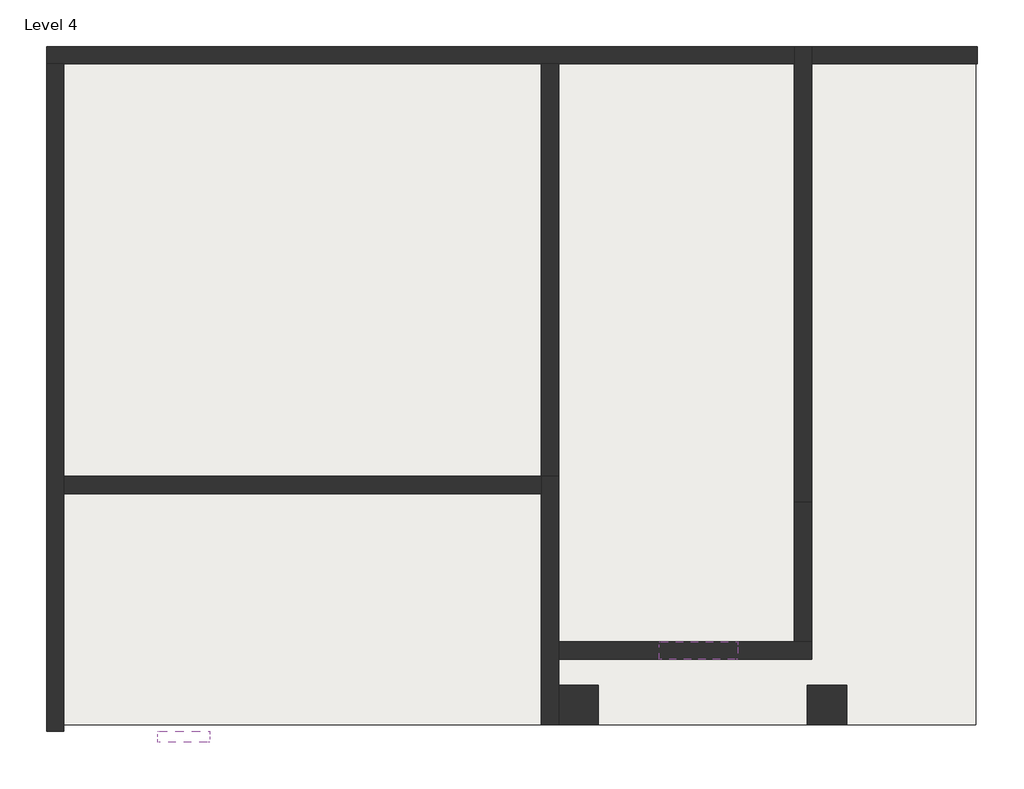
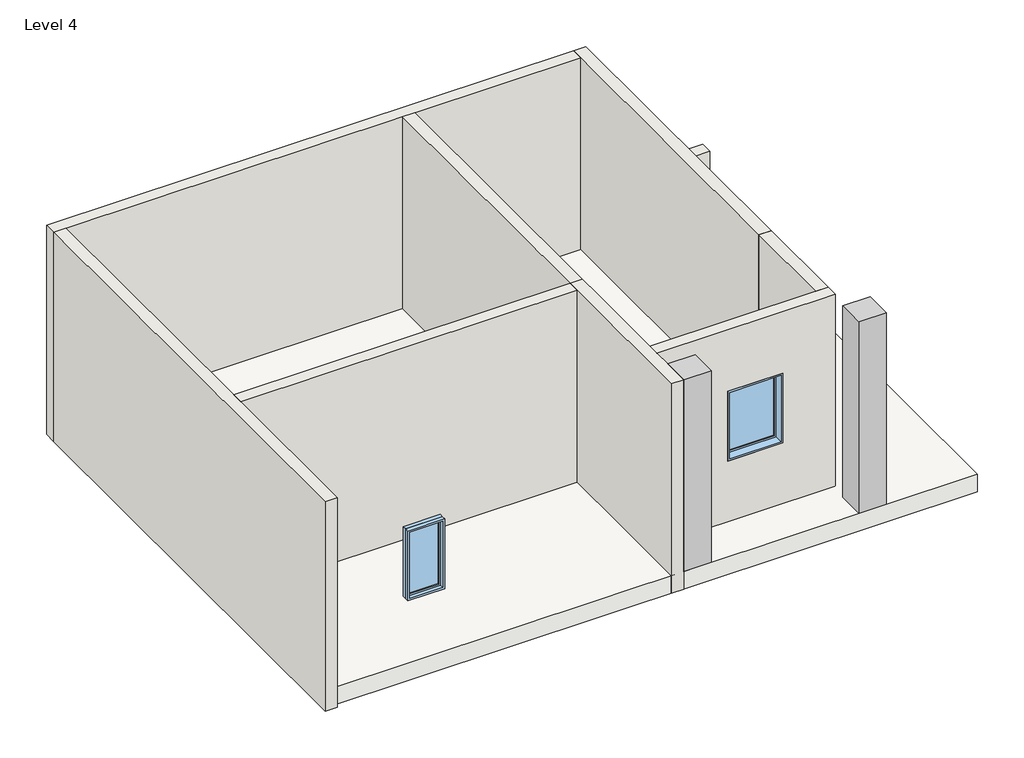
# One storey: 9 walls, 2 columns, 2 windows, 1 roof.
"""IFC4 building model written with IfcOpenShell, lengths in millimetres."""

from ifc_helpers import new_model, si_unit, frame, origin, place, context, project, spatial, polyline, outline, extrude, faceted_brep, transform, mapped, element, save
from components import window_4879aceb, window_e2841890

model = new_model("IFC4")

# Units and contexts
model_context = context("Model", 3, world=origin())
ifc_project = project(units=[si_unit("LENGTHUNIT", "METRE", prefix="MILLI")], contexts=[model_context])

# Site, building, storey
site = spatial("IfcSite", under=ifc_project)
building = spatial("IfcBuilding", under=site)
storey = spatial("IfcBuildingStorey", under=building, Name="Level 4", Elevation=10972.8)

# Columns
placement = place(None, origin())
element("IfcColumn", 1, ObjectType="Rectangular Column : 18\" x 18\"", at=placement, inside=storey, context=model_context, shape_type="SweptSolid", body=[
    extrude(outline(polyline([(-4893.9304753, 3516.0297737), (-4893.9304753, 3058.8297737), (-5351.1304753, 3058.8297737), (-5351.1304753, 3516.0297737), (-4893.9304753, 3516.0297737)])), frame((0.0, 0.0, 11277.6), z_axis=(0.0, 0.0, 1.0), x_axis=(1.0, 0.0, 0.0)), (0.0, 0.0, 1.0), 3352.8),
])
element("IfcColumn", 2, ObjectType="Rectangular Column : 18\" x 18\"", at=placement, inside=storey, context=model_context, shape_type="SweptSolid", body=[
    extrude(outline(polyline([(-7789.5304753, 3516.0297737), (-7789.5304753, 3058.8297737), (-8246.7304753, 3058.8297737), (-8246.7304753, 3516.0297737), (-7789.5304753, 3516.0297737)])), frame((0.0, 0.0, 11277.6), z_axis=(0.0, 0.0, 1.0), x_axis=(1.0, 0.0, 0.0)), (0.0, 0.0, 1.0), 3352.8),
])

# Roof
element("IfcRoof", 3, ObjectType="Generic - 12\"", at=placement, inside=storey, context=model_context, shape_type="SweptSolid", body=[
    extrude(outline(polyline([(-14209.7864811, 10932.8297737), (-3389.3864811, 10932.8297737), (-3389.3864811, 3058.8297737), (-14209.7864811, 3058.8297737), (-14209.7864811, 10932.8297737)])), frame((0.0, 0.0, 10972.8), z_axis=(0.0, 0.0, 1.0), x_axis=(1.0, 0.0, 0.0)), (0.0, 0.0, 1.0), 304.8),
])

# Walls
element("IfcWall", 4, ObjectType="Generic - 8\"", at=placement, inside=storey, context=model_context, shape_type="Brep", body=[
    faceted_brep([(-8449.9304753, 5955.2732783, 10972.8), (-8449.9304753, 5752.0732783, 10972.8), (-8449.9304753, 5548.8732783, 10972.8), (-8449.9304753, 3058.8297737, 10972.8), (-8449.9304753, 3058.8297737, 14630.4), (-8449.9304753, 5548.8732783, 14630.4), (-8449.9304753, 5752.0732783, 14630.4), (-8449.9304753, 5955.2732783, 14630.4), (-8246.7304753, 5955.2732783, 10972.8), (-8246.7304753, 5955.2732783, 14630.4), (-8246.7304753, 5548.8732783, 14630.4), (-8246.7304753, 4024.0297737, 14630.4), (-8246.7304753, 3820.8297737, 14630.4), (-8246.7304753, 3516.0297737, 14630.4), (-8246.7304753, 3058.8297737, 14630.4), (-8246.7304753, 3058.8297737, 11277.6), (-8246.7304753, 3058.8297737, 10972.8), (-8246.7304753, 3820.8297737, 10972.8), (-8246.7304753, 4024.0297737, 10972.8), (-8246.7304753, 5548.8732783, 10972.8)], [[[0, 1, 2, 3, 4, 5, 6, 7]], [[8, 9, 10, 11, 12, 13, 14, 15, 16, 17, 18, 19]], [[3, 2, 1, 0, 8, 19, 18, 17, 16]], [[7, 6, 5, 4, 14, 13, 12, 11, 10, 9]], [[4, 3, 16, 15, 14]], [[0, 7, 9, 8]]]),
])
element("IfcWall", 5, ObjectType="Generic - 8\"", at=placement, inside=storey, context=model_context, shape_type="Brep", body=[
    faceted_brep([(-5300.3304753, 5650.4732783, 10972.8), (-5300.3304753, 10958.2297737, 10972.8), (-5300.3304753, 10958.2297737, 11259.6125244), (-5300.3304753, 10958.2297737, 12248.4392493), (-5300.3304753, 10958.2297737, 14630.4), (-5300.3304753, 5650.4732783, 14630.4), (-5503.5304753, 5650.4732783, 10972.8), (-5503.5304753, 5650.4732783, 14630.4), (-5503.5304753, 10755.0297737, 14630.4), (-5503.5304753, 10958.2297737, 14630.4), (-5503.5304753, 10958.2297737, 10972.8), (-5503.5304753, 10755.0297737, 10972.8)], [[[0, 1, 2, 3, 4, 5]], [[6, 7, 8, 9, 10, 11]], [[1, 0, 6, 11, 10]], [[5, 4, 9, 8, 7]], [[0, 5, 7, 6]], [[1, 10, 9, 4, 3, 2]]]),
])
element("IfcWall", 6, ObjectType="Generic - 8\"", at=placement, inside=storey, context=model_context, shape_type="Brep", body=[
    faceted_brep([(-5503.5304753, 10958.2297737, 14630.4), (-5503.5304753, 10958.2297737, 10972.8), (-14212.6992777, 10958.2297737, 10972.8), (-14212.6992777, 10958.2297737, 14630.4), (-5503.5304753, 10755.0297737, 10972.8), (-5503.5304753, 10755.0297737, 14630.4), (-8246.7304753, 10755.0297737, 14630.4), (-8449.9304753, 10755.0297737, 14630.4), (-14009.4992777, 10755.0297737, 14630.4), (-14212.6992777, 10755.0297737, 14630.4), (-14212.6992777, 10755.0297737, 10972.8), (-14009.4992777, 10755.0297737, 10972.8), (-8449.9304753, 10755.0297737, 10972.8), (-8246.7304753, 10755.0297737, 10972.8)], [[[0, 1, 2, 3]], [[4, 5, 6, 7, 8, 9, 10, 11, 12, 13]], [[2, 1, 4, 13, 12, 11, 10]], [[0, 3, 9, 8, 7, 6, 5]], [[3, 2, 10, 9]], [[0, 5, 4, 1]]]),
])
element("IfcWall", 7, ObjectType="Generic - 8\"", at=placement, inside=storey, context=model_context, shape_type="Brep", body=[
    faceted_brep([(-14212.6992777, 10755.0297737, 10972.8), (-14212.6992777, 2982.6297737, 10972.8), (-14212.6992777, 2982.6297737, 14630.4), (-14212.6992777, 10755.0297737, 14630.4), (-14009.4992777, 10755.0297737, 10972.8), (-14009.4992777, 10755.0297737, 14630.4), (-14009.4992777, 5955.2732783, 14630.4), (-14009.4992777, 5752.0732783, 14630.4), (-14009.4992777, 2982.6297737, 14630.4), (-14009.4992777, 2982.6297737, 10972.8), (-14009.4992777, 5752.0732783, 10972.8), (-14009.4992777, 5955.2732783, 10972.8)], [[[0, 1, 2, 3]], [[4, 5, 6, 7, 8, 9, 10, 11]], [[1, 0, 4, 11, 10, 9]], [[3, 2, 8, 7, 6, 5]], [[0, 3, 5, 4]], [[2, 1, 9, 8]]]),
])
element("IfcWall", 8, ObjectType="Generic - 8\"", at=placement, inside=storey, context=model_context, shape_type="SweptSolid", body=[
    extrude(outline(polyline([(-3369.9304753, 10755.0297737), (-5300.3304753, 10755.0297737), (-5300.3304753, 10958.2297737), (-3369.9304753, 10958.2297737), (-3369.9304753, 10755.0297737)])), frame((0.0, 0.0, 11259.6125244), z_axis=(0.0, 0.0, 1.0), x_axis=(1.0, 0.0, 0.0)), (0.0, 0.0, 1.0), 988.8267249),
])
element("IfcWall", 9, ObjectType="Generic - 8\"", at=placement, inside=storey, context=model_context, shape_type="Brep", body=[
    faceted_brep([(-8246.7304753, 3820.8297737, 10972.8), (-5300.3304753, 3820.8297737, 10972.8), (-5300.3304753, 3820.8297737, 14630.4), (-8246.7304753, 3820.8297737, 14630.4), (-6163.9304753, 3820.8297737, 13556.4516796), (-6163.9304753, 3820.8297737, 12337.2516796), (-7078.3304753, 3820.8297737, 12337.2516796), (-7078.3304753, 3820.8297737, 13556.4516796), (-8246.7304753, 4024.0297737, 10972.8), (-8246.7304753, 4024.0297737, 14630.4), (-5503.5304753, 4024.0297737, 14630.4), (-5300.3304753, 4024.0297737, 14630.4), (-5300.3304753, 4024.0297737, 10972.8), (-5503.5304753, 4024.0297737, 10972.8), (-6163.9304753, 4024.0297737, 13556.4516796), (-7078.3304753, 4024.0297737, 13556.4516796), (-7078.3304753, 4024.0297737, 12337.2516796), (-6163.9304753, 4024.0297737, 12337.2516796)], [[[0, 1, 2, 3], [4, 5, 6, 7]], [[8, 9, 10, 11, 12, 13], [14, 15, 16, 17]], [[1, 0, 8, 13, 12]], [[3, 2, 11, 10, 9]], [[0, 3, 9, 8]], [[2, 1, 12, 11]], [[5, 4, 14, 17]], [[6, 5, 17, 16]], [[7, 6, 16, 15]], [[4, 7, 15, 14]]]),
])
element("IfcWall", 10, ObjectType="Generic - 8\"", at=placement, inside=storey, context=model_context, shape_type="SweptSolid", body=[
    extrude(outline(polyline([(-5503.5304753, 4024.0297737), (-5503.5304753, 5650.4732783), (-5300.3304753, 5650.4732783), (-5300.3304753, 4024.0297737), (-5503.5304753, 4024.0297737)])), frame((0.0, 0.0, 10972.8), z_axis=(0.0, 0.0, 1.0), x_axis=(1.0, 0.0, 0.0)), (0.0, 0.0, 1.0), 3657.6),
])
element("IfcWall", 11, ObjectType="Generic - 8\"", at=placement, inside=storey, context=model_context, shape_type="SweptSolid", body=[
    extrude(outline(polyline([(-14009.4992777, 5955.2732783), (-8449.9304753, 5955.2732783), (-8449.9304753, 5752.0732783), (-14009.4992777, 5752.0732783), (-14009.4992777, 5955.2732783)])), frame((0.0, 0.0, 10972.8), z_axis=(0.0, 0.0, 1.0), x_axis=(1.0, 0.0, 0.0)), (0.0, 0.0, 1.0), 3657.6),
])
element("IfcWall", 12, ObjectType="Generic - 8\"", at=placement, inside=storey, context=model_context, shape_type="SweptSolid", body=[
    extrude(outline(polyline([(-8246.7304753, 10755.0297737), (-8246.7304753, 5955.2732783), (-8449.9304753, 5955.2732783), (-8449.9304753, 10755.0297737), (-8246.7304753, 10755.0297737)])), frame((0.0, 0.0, 10972.8), z_axis=(0.0, 0.0, 1.0), x_axis=(1.0, 0.0, 0.0)), (0.0, 0.0, 1.0), 3657.6),
])

# Windows
window_shape = window_4879aceb(model_context)
element("IfcWindow", 13, ObjectType="Fixed : 24\" x 48\"", at=placement, inside=storey, context=model_context, shape_type="MappedRepresentation", body=[
    mapped(window_shape, transform((-12577.4304753, 2919.1297737, 11613.4331892), x_axis=(1.0, 0.0, 0.0), y_axis=(0.0, 1.0, 0.0), z_axis=(0.0, 0.0, 1.0))),
])
window_2_shape = window_e2841890(model_context)
element("IfcWindow", 14, ObjectType="Fixed : 36\" x 48\"", at=placement, inside=storey, context=model_context, shape_type="MappedRepresentation", body=[
    mapped(window_2_shape, transform((-6583.0304753, 3922.4297737, 11422.8516796), x_axis=(1.0, 0.0, 0.0), y_axis=(0.0, 1.0, 0.0), z_axis=(0.0, 0.0, 1.0))),
])

save(model, "model.ifc")

# Revit data of these elements
# Type "Rectangular Column : 18\" x 18\""
#   Assembly Code = "B1010200"
#   Depth = 1' - 6"
#   Offset Base = 0' - 0"
#   Offset Top = 0' - 0"
#   Width = 1' - 6"
#   Material = none
# Type "Generic - 12\""
#   Assembly Code = "B1020"
#   Layers, outside or top first: 1' - 0" no material (function 1)
# Type "Generic - 8\""
#   Assembly Code = "B2010"
#   Layers, outside or top first: 0' - 8" no material (function 1)
# Type "Fixed : 24\" x 48\""
#   Type Mark = "2"
#   Construction Type Id = "GSP4R"
#   Assembly Code = "B2020100"
#   Analytic Construction = "1/8 in Pilkington single glazing"
#   Visual Light Transmittance = 0.9
#   Solar Heat Gain Coefficient = 0.78
#   Heat Transfer Coefficient (U) = 0.6496 BTU/(h·ft²·°F)
#   Height = 4' - 0"
#   Default Sill Height = 3' - 0"
#   Width = 2' - 0"
#   Window Inset = 0' - 0 3/4"
#   Define Thermal Properties by = 1
#   Glass Pane Material = Glass
#   Sash Material = Sash
#   Wall Closure = (empty or 0)
# Type "Fixed : 36\" x 48\""
#   Type Mark = "1"
#   Construction Type Id = "GSP4R"
#   Assembly Code = "B2020100"
#   Analytic Construction = "1/8 in Pilkington single glazing"
#   Visual Light Transmittance = 0.9
#   Solar Heat Gain Coefficient = 0.78
#   Heat Transfer Coefficient (U) = 0.6496 BTU/(h·ft²·°F)
#   Height = 4' - 0"
#   Default Sill Height = 3' - 0"
#   Width = 3' - 0"
#   Window Inset = 0' - 0 3/4"
#   Define Thermal Properties by = 1
#   Glass Pane Material = Glass
#   Sash Material = Sash
#   Wall Closure = (empty or 0)
# Element 1 (IfcColumn, "Rectangular Column : 18\" x 18\"")
#   Phase Created = New Construction
# Element 2 (IfcColumn, "Rectangular Column : 18\" x 18\"")
#   Phase Created = New Construction
#   Materials on its faces: "Default Wall"
# Element 3 (IfcRoof, "Generic - 12\"")
#   built-in parameter 1001705 = 37 (stored number, unit not read)
#   built-in parameter 1001710 = 33615
#   Phase Created = New Construction
#   Materials on its faces: "Default Roof"
# Elements 4, 5, 6, 7, 9, 10, 11, 12 (IfcWall, "Generic - 8\"")
#   Top Offset = 0' - 0"
#   Base Offset = 0' - 0"
#   Unconnected Height = 12' - 0"
#   wall height = 12' - 0"
#   Phase Created = New Construction
#   Base Constraint = Level 4
#   Materials on its faces: "Default Wall"
# Element 8 (IfcWall, "Generic - 8\"")
#   built-in parameter 1001111 = 0' - 11.29183"
#   Top Offset = 0' - 0"
#   Base Offset = 0' - 11.29183"
#   Unconnected Height = 3' - 2.93019"
#   wall height = 3' - 2.93019"
#   Phase Created = New Construction
#   Base Constraint = Level 4
#   Materials on its faces: "Default Wall"
# Element 13 (IfcWindow, "Fixed : 24\" x 48\"")
#   Mark = "6"
#   Phase Created = New Construction
#   Materials on its faces: "Sash", "Glass"
# Element 14 (IfcWindow, "Fixed : 36\" x 48\"")
#   Mark = "1"
#   Phase Created = New Construction
#   Materials on its faces: "Sash", "Glass"
# Materials
#   "Glass": class "Glass", colour RGB 0 128 192, transparency 0.75, Description = "Soda Lime Glass", Cost = 0
#   "Sash": class "Wood", colour RGB 224 178 126, transparency 0
#   "Default Wall": colour RGB 128 128 128, transparency 0
#   "Default Roof": colour RGB 88 101 114, transparency 0
